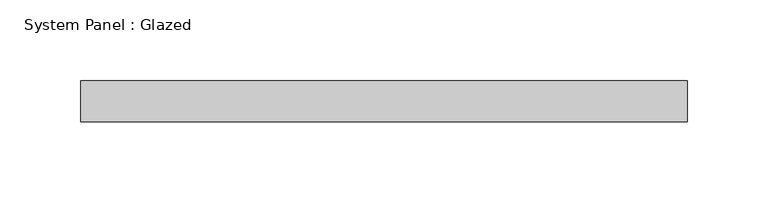
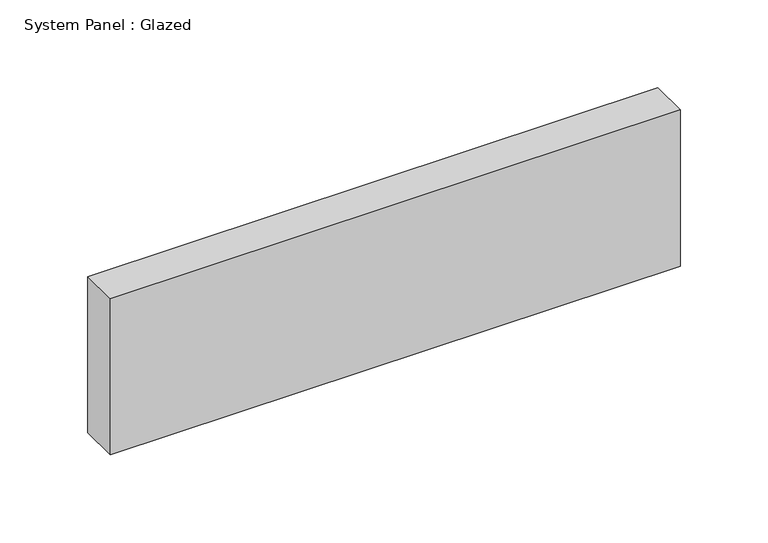
"""IFC4 building model written with IfcOpenShell, lengths in millimetres: plate geometry, System Panel : Glazed."""

from ifc_helpers import new_model, si_unit, origin, origin_with_axes, place, context, project, spatial, polyline, outline, extrude, source, transform, mapped, element, save


def system_panel_glazed_ac390e92(model_context):
    return source(origin(), model_context, "Body", "SweptSolid", [
        extrude(outline(polyline([(187.5766464, 19.05), (-187.5766464, 19.05), (-187.5766464, 44.45), (187.5766464, 44.45), (187.5766464, 19.05)])), origin_with_axes(), (0.0, 0.0, 1.0), 108.6326151),
    ])


if __name__ == "__main__":
    model = new_model("IFC4")
    model_context = context("Model", 3, world=origin())
    ifc_project = project(units=[si_unit("LENGTHUNIT", "METRE", prefix="MILLI")], contexts=[model_context])
    site = spatial("IfcSite", under=ifc_project)
    building = spatial("IfcBuilding", under=site)
    placement = place(None, origin())
    system_panel_glazed_shape = system_panel_glazed_ac390e92(model_context)
    element("IfcPlate", 1, ObjectType="System Panel : Glazed", at=placement, inside=building, context=model_context, shape_type="MappedRepresentation", body=[
        mapped(system_panel_glazed_shape, transform((0.0, 0.0, 0.0), x_axis=(1.0, 0.0, 0.0), y_axis=(0.0, 1.0, 0.0), z_axis=(0.0, 0.0, 1.0))),
    ])
    save(model, "model.ifc")

# Revit data of these elements
# Type "System Panel : Glazed"
#   Construction Type Id = "GSP4R"
#   Analytic Construction = "1/8 in Pilkington single glazing"
#   Visual Light Transmittance = 0.9
#   Solar Heat Gain Coefficient = 0.86
#   Heat Transfer Coefficient (U) = 1.18115 BTU/(h·ft²·°F)
#   Define Thermal Properties by = 1
# Element 1 (IfcPlate, "System Panel : Glazed")
#   Materials on its faces: "Glass"
# Materials
#   "Glass": class "Glass", colour RGB 0 128 192, transparency 0.75, Description = "Soda Lime Glass", Cost = 0
